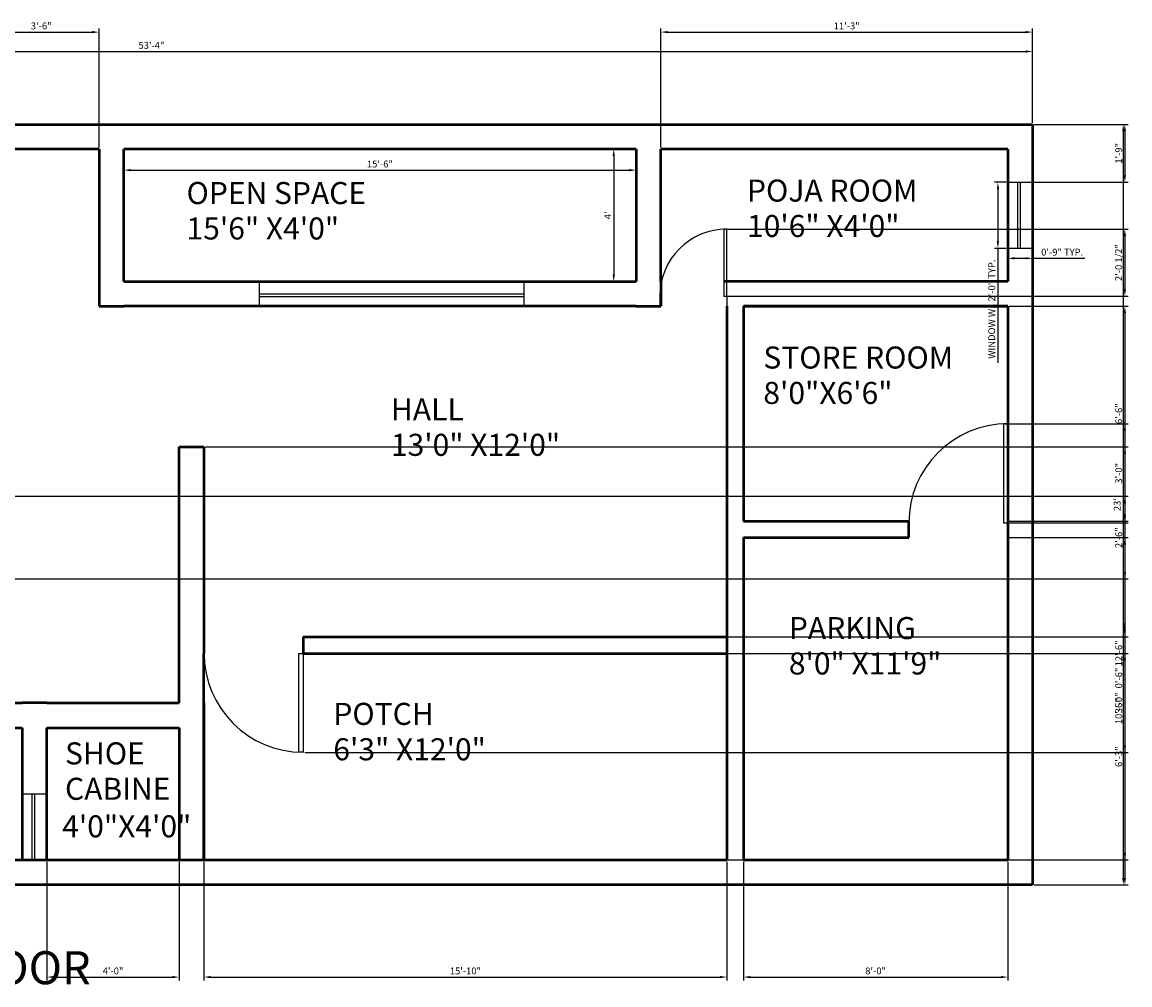
# Model space of a CAD drawing. Units: inches. Extents: x -5798 to 2718, y 1530 to 38999.
# Tile 4 of 4: x 2316 to 2718, y 1990 to 2339. Entities that reach past the tile are written whole.
import ezdxf

# ---------------------------------------------------------------- set-up
doc = ezdxf.new("R2010")
doc.units = ezdxf.units.IN
for name, color, linetype, lineweight in [('A-ANNO-DIMS', 2, 'Continuous', 18), ('A-ANNO-TEXT', 7, 'Continuous', 25), ('A-AREA-IDEN', 3, 'Continuous', 18), ('A-DOOR', 3, 'Continuous', 25), ('A-GLAZ', 4, 'Continuous', 25), ('A-WALL', 7, 'Continuous', 50)]:
    doc.layers.add(name, color=color, linetype=linetype, lineweight=lineweight)
doc.styles.get("Standard").update_dxf_attribs({"font": 'arial.ttf'})
doc.dimstyles.new('Copy of ISO-25', dxfattribs={"dimtxt": 2.5, "dimasz": 2.5, "dimexe": 1.25, "dimexo": 0.625, "dimtad": 1, "dimdec": 1, "dimlunit": 4, "dimtxsty": 'Standard', "dimcen": 2.5, "dimadec": 0, "dimazin": 0, "dimtfac": 1, "dimtdec": 1, "dimtmove": 0, "dimatfit": 3, "dimfxl": 1, "dimarcsym": 0})

# ---------------------------------------------------------------- blocks, each defined once
blk = doc.blocks.new('*U6')
for p, q in [((-40, 0), (-40, 6)), ((0, 0), (0, 6))]:
    blk.add_line(p, q)
blk.add_lwpolyline([(0, 0), (0, -40), (-1.75, -40), (-1.75, 0)], close=True)
blk.add_arc((0, 0), 40, 180, 270)
blk = doc.blocks.new('*U5')
for p, q in [((0, 0), (0, -6)), ((-40, 0), (-40, -6))]:
    blk.add_line(p, q)
blk.add_lwpolyline([(0, 0), (0, 40), (-1.75, 40), (-1.75, 0)], close=True)
blk.add_arc((0, 0), 40, 90, 180)
blk = doc.blocks.new('*D9')
at = {"layer": 'A-ANNO-DIMS', "color": 0, "lineweight": -2, "transparency": 16777216}
for p, q in [((2352.89, 2292.65), (2352.89, 2284.42)), ((2538.89, 2292.65), (2538.89, 2284.42)), ((2355.39, 2285.67), (2536.39, 2285.67))]:
    blk.add_line(p, q, dxfattribs=at)
at = {"layer": 'A-ANNO-DIMS', "color": 0, "transparency": 16777216}
for points in [[(2355.39, 2286.09), (2355.39, 2285.25), (2352.89, 2285.67)], [(2536.39, 2286.09), (2536.39, 2285.25), (2538.89, 2285.67)]]:
    blk.add_solid(points, dxfattribs=at)
at = {"layer": 'Defpoints', "color": 0, "transparency": 16777216}
for p in [(2352.89, 2293.28), (2538.89, 2293.28), (2538.89, 2285.67)]:
    blk.add_point(p, dxfattribs=at)
at = {"layer": 'A-ANNO-DIMS', "color": 0, "transparency": 16777216, "insert": (2445.89, 2287.57), "char_height": 2.5, "attachment_point": 5}
blk.add_mtext('15\'-6"', dxfattribs=at)
blk = doc.blocks.new('*D10')
at = {"layer": 'A-ANNO-DIMS', "color": 0, "lineweight": -2, "transparency": 16777216}
for p, q in [((2538.27, 2293.28), (2529.55, 2293.28)), ((2530.8, 2290.78), (2530.8, 2247.78)), ((2538.27, 2245.28), (2529.55, 2245.28))]:
    blk.add_line(p, q, dxfattribs=at)
at = {"layer": 'A-ANNO-DIMS', "color": 0, "transparency": 16777216}
for points in [[(2530.38, 2290.78), (2531.21, 2290.78), (2530.8, 2293.28)], [(2530.38, 2247.78), (2531.21, 2247.78), (2530.8, 2245.28)]]:
    blk.add_solid(points, dxfattribs=at)
at = {"layer": 'Defpoints', "color": 0, "transparency": 16777216}
for p in [(2538.89, 2293.28), (2530.8, 2245.28), (2538.89, 2245.28)]:
    blk.add_point(p, dxfattribs=at)
at = {"layer": 'A-ANNO-DIMS', "color": 0, "transparency": 16777216, "insert": (2528.92, 2269.28), "char_height": 2.5, "attachment_point": 5, "rotation": 90}
blk.add_mtext("4'", dxfattribs=at)
blk = doc.blocks.new('*D13')
at = {"layer": 'A-ANNO-DIMS', "color": 0, "lineweight": -2, "transparency": 16777216}
for p, q in [((2042.98, 2302.9), (2042.98, 2329.99)), ((2682.89, 2302.9), (2682.89, 2329.99)), ((2045.48, 2328.74), (2680.39, 2328.74))]:
    blk.add_line(p, q, dxfattribs=at)
at = {"layer": 'A-ANNO-DIMS', "color": 0, "transparency": 16777216}
for points in [[(2045.48, 2329.16), (2045.48, 2328.32), (2042.98, 2328.74)], [(2680.39, 2329.16), (2680.39, 2328.32), (2682.89, 2328.74)]]:
    blk.add_solid(points, dxfattribs=at)
at = {"layer": 'Defpoints', "color": 0, "transparency": 16777216}
for p in [(2682.89, 2328.74), (2042.98, 2302.28), (2682.89, 2302.28)]:
    blk.add_point(p, dxfattribs=at)
at = {"layer": 'A-ANNO-DIMS', "color": 0, "transparency": 16777216, "insert": (2362.93, 2330.64), "char_height": 2.5, "attachment_point": 5}
blk.add_mtext('53\'-4"', dxfattribs=at)
blk = doc.blocks.new('*D14')
at = {"layer": 'A-ANNO-DIMS', "color": 0, "lineweight": -2, "transparency": 16777216}
for p, q in [((2683.52, 2302.28), (2717.07, 2302.28)), ((2715.82, 2299.78), (2715.82, 2028.78)), ((2683.52, 2026.28), (2717.07, 2026.28))]:
    blk.add_line(p, q, dxfattribs=at)
at = {"layer": 'A-ANNO-DIMS', "color": 0, "transparency": 16777216}
for points in [[(2715.4, 2299.78), (2716.23, 2299.78), (2715.82, 2302.28)], [(2715.4, 2028.78), (2716.23, 2028.78), (2715.82, 2026.28)]]:
    blk.add_solid(points, dxfattribs=at)
at = {"layer": 'Defpoints', "color": 0, "transparency": 16777216}
for p in [(2682.89, 2302.28), (2682.89, 2026.28), (2715.82, 2026.28)]:
    blk.add_point(p, dxfattribs=at)
at = {"layer": 'A-ANNO-DIMS', "color": 0, "transparency": 16777216, "insert": (2713.92, 2164.28), "char_height": 2.5, "attachment_point": 5, "rotation": 90}
blk.add_mtext("23'", dxfattribs=at)
blk = doc.blocks.new('WIN-24')
for p, q in [((0, 0), (0, 9)), ((0, 9), (24, 9)), ((24, 9), (24, 0)), ((0, 4.5), (24, 4.5)), ((0, 3.5), (24, 3.5))]:
    blk.add_line(p, q)
blk = doc.blocks.new('*D22')
at = {"layer": 'A-ANNO-DIMS', "color": 0, "lineweight": -2, "transparency": 16777216}
for p, q in [((2673.27, 2281.28), (2669.04, 2281.28)), ((2670.29, 2278.78), (2670.29, 2259.78)), ((2673.27, 2257.28), (2669.04, 2257.28)), ((2670.29, 2257.28), (2670.29, 2215.68))]:
    blk.add_line(p, q, dxfattribs=at)
at = {"layer": 'A-ANNO-DIMS', "color": 0, "transparency": 16777216}
for points in [[(2669.88, 2278.78), (2670.71, 2278.78), (2670.29, 2281.28)], [(2669.88, 2259.78), (2670.71, 2259.78), (2670.29, 2257.28)]]:
    blk.add_solid(points, dxfattribs=at)
at = {"layer": 'Defpoints', "color": 0, "transparency": 16777216}
for p in [(2673.89, 2281.28), (2670.29, 2257.28), (2673.89, 2257.28)]:
    blk.add_point(p, dxfattribs=at)
at = {"layer": 'A-ANNO-DIMS', "color": 0, "transparency": 16777216, "insert": (2668.38, 2235.23), "char_height": 2.5, "attachment_point": 5, "rotation": 90}
blk.add_mtext('WINDOW W1 2\'-0" TYP.', dxfattribs=at)
blk = doc.blocks.new('*D23')
at = {"layer": 'A-ANNO-DIMS', "color": 0, "lineweight": -2, "transparency": 16777216}
for p, q in [((2673.89, 2256.65), (2673.89, 2252.43)), ((2682.89, 2256.65), (2682.89, 2252.43)), ((2676.39, 2253.68), (2680.39, 2253.68)), ((2682.89, 2253.68), (2701.88, 2253.68))]:
    blk.add_line(p, q, dxfattribs=at)
at = {"layer": 'A-ANNO-DIMS', "color": 0, "transparency": 16777216}
for points in [[(2676.39, 2254.09), (2676.39, 2253.26), (2673.89, 2253.68)], [(2680.39, 2254.09), (2680.39, 2253.26), (2682.89, 2253.68)]]:
    blk.add_solid(points, dxfattribs=at)
at = {"layer": 'Defpoints', "color": 0, "transparency": 16777216}
for p in [(2673.89, 2257.28), (2682.89, 2257.28), (2682.89, 2253.68)]:
    blk.add_point(p, dxfattribs=at)
at = {"layer": 'A-ANNO-DIMS', "color": 0, "transparency": 16777216, "insert": (2693.64, 2255.58), "char_height": 2.5, "attachment_point": 5}
blk.add_mtext('0\'-9" TYP.', dxfattribs=at)
blk = doc.blocks.new('*D37')
at = {"layer": 'A-ANNO-DIMS', "color": 0, "lineweight": -2, "transparency": 16777216}
for p, q in [((2301.89, 2293.9), (2301.89, 2337.03)), ((2343.89, 2293.9), (2343.89, 2337.03)), ((2304.39, 2335.78), (2341.39, 2335.78))]:
    blk.add_line(p, q, dxfattribs=at)
at = {"layer": 'A-ANNO-DIMS', "color": 0, "transparency": 16777216}
for points in [[(2304.39, 2336.19), (2304.39, 2335.36), (2301.89, 2335.78)], [(2341.39, 2336.19), (2341.39, 2335.36), (2343.89, 2335.78)]]:
    blk.add_solid(points, dxfattribs=at)
at = {"layer": 'Defpoints', "color": 0, "transparency": 16777216}
for p in [(2343.89, 2335.78), (2301.89, 2293.28), (2343.89, 2293.28)]:
    blk.add_point(p, dxfattribs=at)
at = {"layer": 'A-ANNO-DIMS', "color": 0, "transparency": 16777216, "insert": (2322.89, 2337.68), "char_height": 2.5, "attachment_point": 5}
blk.add_mtext('3\'-6"', dxfattribs=at)
blk = doc.blocks.new('*D38')
at = {"layer": 'A-ANNO-DIMS', "color": 0, "lineweight": -2, "transparency": 16777216}
for p, q in [((2547.89, 2293.9), (2547.89, 2337.03)), ((2682.89, 2302.9), (2682.89, 2337.03)), ((2550.39, 2335.78), (2680.39, 2335.78))]:
    blk.add_line(p, q, dxfattribs=at)
at = {"layer": 'A-ANNO-DIMS', "color": 0, "transparency": 16777216}
for points in [[(2550.39, 2336.19), (2550.39, 2335.36), (2547.89, 2335.78)], [(2680.39, 2336.19), (2680.39, 2335.36), (2682.89, 2335.78)]]:
    blk.add_solid(points, dxfattribs=at)
at = {"layer": 'Defpoints', "color": 0, "transparency": 16777216}
for p in [(2682.89, 2335.78), (2682.89, 2302.28), (2547.89, 2293.28)]:
    blk.add_point(p, dxfattribs=at)
at = {"layer": 'A-ANNO-DIMS', "color": 0, "transparency": 16777216, "insert": (2615.39, 2337.68), "char_height": 2.5, "attachment_point": 5}
blk.add_mtext('11\'-3"', dxfattribs=at)
blk = doc.blocks.new('*D44')
at = {"layer": 'A-ANNO-DIMS', "color": 0, "lineweight": -2, "transparency": 16777216}
for p, q in [((2683.52, 2302.28), (2717.64, 2302.28)), ((2716.39, 2299.78), (2716.39, 2283.78)), ((2683.52, 2281.28), (2717.64, 2281.28))]:
    blk.add_line(p, q, dxfattribs=at)
at = {"layer": 'A-ANNO-DIMS', "color": 0, "transparency": 16777216}
for points in [[(2715.98, 2299.78), (2716.81, 2299.78), (2716.39, 2302.28)], [(2715.98, 2283.78), (2716.81, 2283.78), (2716.39, 2281.28)]]:
    blk.add_solid(points, dxfattribs=at)
at = {"layer": 'Defpoints', "color": 0, "transparency": 16777216}
for p in [(2682.89, 2302.28), (2682.89, 2281.28), (2716.39, 2281.28)]:
    blk.add_point(p, dxfattribs=at)
at = {"layer": 'A-ANNO-DIMS', "color": 0, "transparency": 16777216, "insert": (2714.49, 2291.78), "char_height": 2.5, "attachment_point": 5, "rotation": 90}
blk.add_mtext('1\'-9"', dxfattribs=at)
blk = doc.blocks.new('*D45')
at = {"layer": 'A-ANNO-DIMS', "color": 0, "lineweight": -2, "transparency": 16777216}
for p, q in [((2674.52, 2236.28), (2717.64, 2236.28)), ((2716.39, 2233.78), (2716.39, 2160.78)), ((2674.52, 2158.28), (2717.64, 2158.28))]:
    blk.add_line(p, q, dxfattribs=at)
at = {"layer": 'A-ANNO-DIMS', "color": 0, "transparency": 16777216}
for points in [[(2715.98, 2233.78), (2716.81, 2233.78), (2716.39, 2236.28)], [(2715.98, 2160.78), (2716.81, 2160.78), (2716.39, 2158.28)]]:
    blk.add_solid(points, dxfattribs=at)
at = {"layer": 'Defpoints', "color": 0, "transparency": 16777216}
for p in [(2673.89, 2236.28), (2673.89, 2158.28), (2716.39, 2158.28)]:
    blk.add_point(p, dxfattribs=at)
at = {"layer": 'A-ANNO-DIMS', "color": 0, "transparency": 16777216, "insert": (2714.49, 2197.28), "char_height": 2.5, "attachment_point": 5, "rotation": 90}
blk.add_mtext('6\'-6"', dxfattribs=at)
blk = doc.blocks.new('*D46')
at = {"layer": 'A-ANNO-DIMS', "color": 0, "lineweight": -2, "transparency": 16777216}
for p, q in [((2674.52, 2152.28), (2717.64, 2152.28)), ((2716.39, 2149.78), (2716.39, 2028.78)), ((2683.52, 2026.28), (2717.64, 2026.28))]:
    blk.add_line(p, q, dxfattribs=at)
at = {"layer": 'A-ANNO-DIMS', "color": 0, "transparency": 16777216}
for points in [[(2715.98, 2149.78), (2716.81, 2149.78), (2716.39, 2152.28)], [(2715.98, 2028.78), (2716.81, 2028.78), (2716.39, 2026.28)]]:
    blk.add_solid(points, dxfattribs=at)
at = {"layer": 'Defpoints', "color": 0, "transparency": 16777216}
for p in [(2673.89, 2152.28), (2682.89, 2026.28), (2716.39, 2026.28)]:
    blk.add_point(p, dxfattribs=at)
at = {"layer": 'A-ANNO-DIMS', "color": 0, "transparency": 16777216, "insert": (2714.49, 2089.28), "char_height": 2.5, "attachment_point": 5, "rotation": 90}
blk.add_mtext('10\'-6"', dxfattribs=at)
blk = doc.blocks.new('*D50')
at = {"layer": 'A-ANNO-DIMS', "color": 0, "lineweight": -2, "transparency": 16777216}
for p, q in [((2324.98, 2034.65), (2324.98, 1991.53)), ((2372.98, 2034.65), (2372.98, 1991.53)), ((2327.48, 1992.78), (2370.48, 1992.78))]:
    blk.add_line(p, q, dxfattribs=at)
at = {"layer": 'A-ANNO-DIMS', "color": 0, "transparency": 16777216}
for points in [[(2327.48, 1993.19), (2327.48, 1992.36), (2324.98, 1992.78)], [(2370.48, 1993.19), (2370.48, 1992.36), (2372.98, 1992.78)]]:
    blk.add_solid(points, dxfattribs=at)
at = {"layer": 'Defpoints', "color": 0, "transparency": 16777216}
for p in [(2324.98, 2035.28), (2372.98, 2035.28), (2372.98, 1992.78)]:
    blk.add_point(p, dxfattribs=at)
at = {"layer": 'A-ANNO-DIMS', "color": 0, "transparency": 16777216, "insert": (2348.98, 1994.68), "char_height": 2.5, "attachment_point": 5}
blk.add_mtext('4\'-0"', dxfattribs=at)
blk = doc.blocks.new('*D51')
at = {"layer": 'A-ANNO-DIMS', "color": 0, "lineweight": -2, "transparency": 16777216}
for p, q in [((2381.98, 2034.65), (2381.98, 1991.53)), ((2571.89, 2034.65), (2571.89, 1991.53)), ((2384.48, 1992.78), (2569.39, 1992.78))]:
    blk.add_line(p, q, dxfattribs=at)
at = {"layer": 'A-ANNO-DIMS', "color": 0, "transparency": 16777216}
for points in [[(2384.48, 1993.19), (2384.48, 1992.36), (2381.98, 1992.78)], [(2569.39, 1993.19), (2569.39, 1992.36), (2571.89, 1992.78)]]:
    blk.add_solid(points, dxfattribs=at)
at = {"layer": 'Defpoints', "color": 0, "transparency": 16777216}
for p in [(2381.98, 2035.28), (2571.89, 2035.28), (2571.89, 1992.78)]:
    blk.add_point(p, dxfattribs=at)
at = {"layer": 'A-ANNO-DIMS', "color": 0, "transparency": 16777216, "insert": (2476.93, 1994.68), "char_height": 2.5, "attachment_point": 5}
blk.add_mtext('15\'-10"', dxfattribs=at)
blk = doc.blocks.new('*D52')
at = {"layer": 'A-ANNO-DIMS', "color": 0, "lineweight": -2, "transparency": 16777216}
for p, q in [((2577.89, 2034.65), (2577.89, 1991.53)), ((2673.89, 2034.65), (2673.89, 1991.53)), ((2580.39, 1992.78), (2671.39, 1992.78))]:
    blk.add_line(p, q, dxfattribs=at)
at = {"layer": 'A-ANNO-DIMS', "color": 0, "transparency": 16777216}
for points in [[(2580.39, 1993.19), (2580.39, 1992.36), (2577.89, 1992.78)], [(2671.39, 1993.19), (2671.39, 1992.36), (2673.89, 1992.78)]]:
    blk.add_solid(points, dxfattribs=at)
at = {"layer": 'Defpoints', "color": 0, "transparency": 16777216}
for p in [(2577.89, 2035.28), (2673.89, 2035.28), (2673.89, 1992.78)]:
    blk.add_point(p, dxfattribs=at)
at = {"layer": 'A-ANNO-DIMS', "color": 0, "transparency": 16777216, "insert": (2625.89, 1994.68), "char_height": 2.5, "attachment_point": 5}
blk.add_mtext('8\'-0"', dxfattribs=at)
blk = doc.blocks.new('*D55')
at = {"layer": 'A-ANNO-DIMS', "color": 0, "lineweight": -2, "transparency": 16777216}
for p, q in [((2382.6, 2185.28), (2717.64, 2185.28)), ((2716.39, 2182.78), (2716.39, 2037.78)), ((2382.6, 2035.28), (2717.64, 2035.28))]:
    blk.add_line(p, q, dxfattribs=at)
at = {"layer": 'A-ANNO-DIMS', "color": 0, "transparency": 16777216}
for points in [[(2715.98, 2182.78), (2716.81, 2182.78), (2716.39, 2185.28)], [(2715.98, 2037.78), (2716.81, 2037.78), (2716.39, 2035.28)]]:
    blk.add_solid(points, dxfattribs=at)
at = {"layer": 'Defpoints', "color": 0, "transparency": 16777216}
for p in [(2381.98, 2185.28), (2381.98, 2035.28), (2716.39, 2035.28)]:
    blk.add_point(p, dxfattribs=at)
at = {"layer": 'A-ANNO-DIMS', "color": 0, "transparency": 16777216, "insert": (2714.49, 2110.28), "char_height": 2.5, "attachment_point": 5, "rotation": 90}
blk.add_mtext('12\'-6"', dxfattribs=at)
blk = doc.blocks.new('*D56')
at = {"layer": 'A-ANNO-DIMS', "color": 0, "lineweight": -2, "transparency": 16777216}
for p, q in [((2572.52, 2110.28), (2717.64, 2110.28)), ((2716.39, 2107.78), (2716.39, 2037.78)), ((2572.52, 2035.28), (2717.64, 2035.28))]:
    blk.add_line(p, q, dxfattribs=at)
at = {"layer": 'A-ANNO-DIMS', "color": 0, "transparency": 16777216}
for points in [[(2715.98, 2107.78), (2716.81, 2107.78), (2716.39, 2110.28)], [(2715.98, 2037.78), (2716.81, 2037.78), (2716.39, 2035.28)]]:
    blk.add_solid(points, dxfattribs=at)
at = {"layer": 'Defpoints', "color": 0, "transparency": 16777216}
for p in [(2571.89, 2110.28), (2571.89, 2035.28), (2716.39, 2035.28)]:
    blk.add_point(p, dxfattribs=at)
at = {"layer": 'A-ANNO-DIMS', "color": 0, "transparency": 16777216, "insert": (2714.49, 2072.78), "char_height": 2.5, "attachment_point": 5, "rotation": 90}
blk.add_mtext('6\'-3"', dxfattribs=at)
blk = doc.blocks.new('*D57')
at = {"layer": 'A-ANNO-DIMS', "color": 0, "lineweight": -2, "transparency": 16777216}
for p, q in [((2716.39, 2118.78), (2716.39, 2121.28)), ((2418.6, 2116.28), (2717.64, 2116.28)), ((2716.39, 2116.28), (2716.39, 2110.28)), ((2418.6, 2110.28), (2717.64, 2110.28)), ((2716.39, 2107.78), (2716.39, 2097.38))]:
    blk.add_line(p, q, dxfattribs=at)
at = {"layer": 'A-ANNO-DIMS', "color": 0, "transparency": 16777216}
for points in [[(2715.98, 2118.78), (2716.81, 2118.78), (2716.39, 2116.28)], [(2715.98, 2107.78), (2716.81, 2107.78), (2716.39, 2110.28)]]:
    blk.add_solid(points, dxfattribs=at)
at = {"layer": 'Defpoints', "color": 0, "transparency": 16777216}
for p in [(2417.98, 2116.28), (2417.98, 2110.28), (2716.39, 2110.28)]:
    blk.add_point(p, dxfattribs=at)
at = {"layer": 'A-ANNO-DIMS', "color": 0, "transparency": 16777216, "insert": (2714.49, 2101.33), "char_height": 2.5, "attachment_point": 5, "rotation": 90}
blk.add_mtext('0\'-6"', dxfattribs=at)
blk = doc.blocks.new('*D59')
at = {"layer": 'A-ANNO-DIMS', "color": 0, "lineweight": -2, "transparency": 16777216}
for p, q in [((2181.6, 2167.28), (2717.64, 2167.28)), ((2716.39, 2164.78), (2716.39, 2139.78)), ((2181.6, 2137.28), (2717.64, 2137.28))]:
    blk.add_line(p, q, dxfattribs=at)
at = {"layer": 'A-ANNO-DIMS', "color": 0, "transparency": 16777216}
for points in [[(2715.98, 2164.78), (2716.81, 2164.78), (2716.39, 2167.28)], [(2715.98, 2139.78), (2716.81, 2139.78), (2716.39, 2137.28)]]:
    blk.add_solid(points, dxfattribs=at)
at = {"layer": 'Defpoints', "color": 0, "transparency": 16777216}
for p in [(2180.98, 2167.28), (2180.98, 2137.28), (2716.39, 2137.28)]:
    blk.add_point(p, dxfattribs=at)
at = {"layer": 'A-ANNO-DIMS', "color": 0, "transparency": 16777216, "insert": (2714.49, 2152.28), "char_height": 2.5, "attachment_point": 5, "rotation": 90}
blk.add_mtext('2\'-6"', dxfattribs=at)
blk = doc.blocks.new('*D62')
at = {"layer": 'A-ANNO-DIMS', "color": 0, "lineweight": -2, "transparency": 16777216}
for p, q in [((2418.6, 2110.28), (2717.64, 2110.28)), ((2716.39, 2107.78), (2716.39, 2076.85)), ((2418.6, 2074.35), (2717.64, 2074.35))]:
    blk.add_line(p, q, dxfattribs=at)
at = {"layer": 'A-ANNO-DIMS', "color": 0, "transparency": 16777216}
for points in [[(2715.98, 2107.78), (2716.81, 2107.78), (2716.39, 2110.28)], [(2715.98, 2076.85), (2716.81, 2076.85), (2716.39, 2074.35)]]:
    blk.add_solid(points, dxfattribs=at)
at = {"layer": 'Defpoints', "color": 0, "transparency": 16777216}
for p in [(2417.98, 2110.28), (2417.98, 2074.35), (2716.39, 2074.35)]:
    blk.add_point(p, dxfattribs=at)
at = {"layer": 'A-ANNO-DIMS', "color": 0, "transparency": 16777216, "insert": (2714.49, 2092.32), "char_height": 2.5, "attachment_point": 5, "rotation": 90}
blk.add_mtext('3\'-0"', dxfattribs=at)
blk = doc.blocks.new('*D63')
at = {"layer": 'A-ANNO-DIMS', "color": 0, "lineweight": -2, "transparency": 16777216}
for p, q in [((2571.45, 2264.3), (2717.64, 2264.3)), ((2716.39, 2261.8), (2716.39, 2242.43)), ((2571.45, 2239.93), (2717.64, 2239.93))]:
    blk.add_line(p, q, dxfattribs=at)
at = {"layer": 'A-ANNO-DIMS', "color": 0, "transparency": 16777216}
for points in [[(2715.98, 2261.8), (2716.81, 2261.8), (2716.39, 2264.3)], [(2715.98, 2242.43), (2716.81, 2242.43), (2716.39, 2239.93)]]:
    blk.add_solid(points, dxfattribs=at)
at = {"layer": 'Defpoints', "color": 0, "transparency": 16777216}
for p in [(2570.83, 2264.3), (2570.83, 2239.93), (2716.39, 2239.93)]:
    blk.add_point(p, dxfattribs=at)
at = {"layer": 'A-ANNO-DIMS', "color": 0, "transparency": 16777216, "insert": (2714.48, 2252.12), "char_height": 2.5, "attachment_point": 5, "rotation": 90}
blk.add_mtext('2\'-0 1/2"', dxfattribs=at)
blk = doc.blocks.new('*D64')
at = {"layer": 'A-ANNO-DIMS', "color": 0, "lineweight": -2, "transparency": 16777216}
for p, q in [((2672.95, 2193.59), (2717.64, 2193.59)), ((2716.39, 2191.09), (2716.39, 2160.17)), ((2672.95, 2157.67), (2717.64, 2157.67))]:
    blk.add_line(p, q, dxfattribs=at)
at = {"layer": 'A-ANNO-DIMS', "color": 0, "transparency": 16777216}
for points in [[(2715.98, 2191.09), (2716.81, 2191.09), (2716.39, 2193.59)], [(2715.98, 2160.17), (2716.81, 2160.17), (2716.39, 2157.67)]]:
    blk.add_solid(points, dxfattribs=at)
at = {"layer": 'Defpoints', "color": 0, "transparency": 16777216}
for p in [(2672.32, 2193.59), (2672.32, 2157.67), (2716.39, 2157.67)]:
    blk.add_point(p, dxfattribs=at)
at = {"layer": 'A-ANNO-DIMS', "color": 0, "transparency": 16777216, "insert": (2714.49, 2175.63), "char_height": 2.5, "attachment_point": 5, "rotation": 90}
blk.add_mtext('3\'-0"', dxfattribs=at)

msp = doc.modelspace()

# ---------------------------------------------------------------- linework, layer by layer
at = {"layer": 'A-GLAZ'}
for p, q in [((2402.14, 2236.28), (2402.14, 2245.28)), ((2498.14, 2245.28), (2498.14, 2236.28)), ((2402.14, 2240.78), (2498.14, 2240.78)), ((2402.14, 2239.78), (2498.14, 2239.78)), ((2498.14, 2236.28), (2402.14, 2236.28))]:
    msp.add_line(p, q, dxfattribs=at)
at = {"layer": 'A-WALL'}
for p, q in [((2301.89, 2302.28), (2541.89, 2302.28)), ((2541.89, 2302.28), (2547.89, 2302.28)), ((2547.89, 2302.28), (2673.89, 2302.28)), ((2673.89, 2302.28), (2682.89, 2302.28)), ((2682.89, 2302.28), (2682.89, 2293.28)), ((2343.89, 2293.28), (2301.89, 2293.28)), ((2343.89, 2293.28), (2343.89, 2245.28)), ((2352.89, 2245.28), (2352.89, 2293.28)), ((2538.89, 2293.28), (2352.89, 2293.28)), ((2538.89, 2293.28), (2538.89, 2245.28)), ((2673.89, 2293.28), (2547.89, 2293.28)), ((2547.89, 2245.28), (2547.89, 2293.28)), ((2673.89, 2293.28), (2673.89, 2245.28)), ((2673.89, 2293.28), (2673.89, 2245.28)), ((2673.89, 2293.28), (2673.89, 2281.28)), ((2682.89, 2293.28), (2682.89, 2245.28)), ((2343.89, 2245.28), (2343.89, 2236.28)), ((2352.89, 2245.28), (2538.89, 2245.28)), ((2498.14, 2245.28), (2498.14, 2245.28)), ((2547.89, 2245.28), (2547.89, 2236.28)), ((2548.12, 2245.28), (2547.89, 2245.28)), ((2673.89, 2245.28), (2570.83, 2245.28)), ((2682.89, 2245.28), (2682.89, 2239.28)), ((2682.89, 2239.28), (2682.89, 2161.28)), ((2343.89, 2236.28), (2352.89, 2236.28)), ((2538.89, 2236.28), (2352.89, 2236.28)), ((2538.89, 2236.28), (2547.89, 2236.28)), ((2571.89, 2236.28), (2571.89, 2158.28)), ((2673.89, 2236.28), (2577.89, 2236.28)), ((2577.89, 2236.28), (2577.89, 2158.28)), ((2577.89, 2236.28), (2673.89, 2236.28)), ((2673.89, 2236.28), (2673.89, 2158.28)), ((2372.98, 2092.28), (2372.98, 2185.28)), ((2372.98, 2185.28), (2381.98, 2185.28)), ((2381.98, 2185.28), (2381.98, 2116.28)), ((2682.89, 2161.28), (2682.89, 2155.28)), ((2571.89, 2158.28), (2571.89, 2152.28)), ((2577.89, 2158.28), (2637.89, 2158.28)), ((2637.89, 2152.28), (2637.89, 2158.28)), ((2673.89, 2158.28), (2673.89, 2152.28)), ((2571.89, 2152.28), (2571.89, 2035.28)), ((2577.89, 2152.28), (2637.89, 2152.28)), ((2577.89, 2152.28), (2577.89, 2035.28)), ((2673.89, 2152.28), (2673.89, 2035.28)), ((2682.89, 2155.28), (2682.89, 2026.28)), ((2381.98, 2118.51), (2381.98, 2118.51)), ((2381.98, 2118.51), (2381.98, 2110.28)), ((2417.98, 2116.28), (2571.89, 2116.28)), ((2417.98, 2116.28), (2417.98, 2110.28)), ((2381.98, 2035.28), (2381.98, 2110.28)), ((2417.98, 2110.28), (2571.89, 2110.28)), ((2278.97, 2092.28), (2315.98, 2092.28)), ((2324.98, 2092.28), (2315.98, 2092.28)), ((2324.98, 2092.28), (2372.98, 2092.28)), ((2381.98, 2092.28), (2381.98, 2035.28)), ((2381.98, 2035.28), (2381.98, 2092.28)), ((2278.97, 2083.28), (2315.98, 2083.28)), ((2315.98, 2083.28), (2315.98, 2035.28)), ((2324.98, 2035.28), (2324.98, 2083.28)), ((2324.98, 2083.28), (2372.98, 2083.28)), ((2372.98, 2083.28), (2372.98, 2035.28)), ((2051.98, 2035.28), (2571.89, 2035.28)), ((2372.98, 2035.28), (2381.98, 2035.28)), ((2577.89, 2035.28), (2673.89, 2035.28)), ((2682.89, 2035.28), (2682.89, 2026.28)), ((2682.89, 2026.28), (2042.98, 2026.28))]:
    msp.add_line(p, q, dxfattribs=at)

# ---------------------------------------------------------------- block references
at = {"layer": 'A-DOOR'}
for name, p, xscale, yscale, zscale in [('*U5', (2571.89, 2239.93), 0.6091863517261157, 0.6091863517261157, 0.6091863517261157), ('*U5', (2673.89, 2157.67), 0.8981214444059173, 0.8981214444059173, 0.8981214444059173), ('*U5', (2673.89, 2157.67), 0.8981214444059173, 0.8981214444059173, 0.8981214444059173), ('*U6', (2417.98, 2110.28), 0.8981214444059173, 0.8981214444059173, 0.8981214444059173)]:
    msp.add_blockref(name, p, dxfattribs=dict(at, xscale=xscale, yscale=yscale, zscale=zscale))
at = {"layer": 'A-GLAZ'}
for p, rotation in [((2673.89, 2281.28), 270.0000000000009), ((2315.98, 2059.28), 269.9999999999973)]:
    msp.add_blockref('WIN-24', p, dxfattribs=dict(at, rotation=rotation))

# ---------------------------------------------------------------- texts
at = {"layer": 'A-ANNO-TEXT'}
msp.add_text('GROUND FLOOR ', height=12, dxfattribs=at).set_placement((2215.86, 1990.17))
at = {"layer": 'A-AREA-IDEN'}
for s, p in [('OPEN SPACE', (2375.66, 2273.36)), ('POJA ROOM', (2579.18, 2274.25)), ('15\'6" X4\'0"', (2375.66, 2260.5)), ('10\'6" X4\'0"', (2579.18, 2261.4)), ('STORE ROOM', (2585.12, 2213.65)), ('8\'0"X6\'6"', (2585.12, 2200.8)), ('HALL', (2449.88, 2194.82)), ('13\'0" X12\'0"', (2449.88, 2181.97)), ('PARKING', (2594.38, 2115.46)), ('8\'0" X11\'9"', (2594.38, 2102.61)), ('POTCH', (2428.97, 2084.31)), ('6\'3" X12\'0"', (2428.97, 2071.46)), ('SHOE', (2331.54, 2069.97)), ('CABINE', (2331.54, 2057.12)), ('4\'0"X4\'0"', (2330.51, 2043.49))]:
    msp.add_text(s, height=8, dxfattribs=at).set_placement(p)

# ---------------------------------------------------------------- dimensions: what is measured, and where the dimension line sits
at = {"layer": 'A-ANNO-DIMS'}
for base, p1, p2, override, picture, middle in [((2343.89, 2335.78), (2301.89, 2293.28), (2343.89, 2293.28), {"dimdec": 1, "dimlfac": 1, "dimrnd": 0, "dimzin": 1, "dimdsep": 46, "dimlunit": 4, "dimfrac": 2}, '*D37', (2322.89, 2337.68)), ((2682.89, 2335.78), (2547.89, 2293.28), (2682.89, 2302.28), {"dimdec": 1, "dimlfac": 1, "dimrnd": 0, "dimzin": 1, "dimdsep": 46, "dimlunit": 4, "dimfrac": 2}, '*D38', (2615.39, 2337.68)), ((2682.89, 2328.74), (2042.98, 2302.28), (2682.89, 2302.28), {"dimclrd": 0, "dimclre": 0, "dimclrt": 0}, '*D13', (2362.93, 2330.64)), ((2538.89, 2285.67), (2352.89, 2293.28), (2538.89, 2293.28), {"dimclrd": 0, "dimclre": 0, "dimclrt": 0}, '*D9', (2445.89, 2287.57)), ((2372.98, 1992.78), (2324.98, 2035.28), (2372.98, 2035.28), {"dimdec": 1, "dimlfac": 1, "dimrnd": 0, "dimzin": 1, "dimdsep": 46, "dimlunit": 4, "dimfrac": 2}, '*D50', (2348.98, 1994.68)), ((2571.89, 1992.78), (2381.98, 2035.28), (2571.89, 2035.28), {"dimdec": 1, "dimlfac": 1, "dimrnd": 0, "dimzin": 1, "dimdsep": 46, "dimlunit": 4, "dimfrac": 2}, '*D51', (2476.93, 1994.68)), ((2673.89, 1992.78), (2577.89, 2035.28), (2673.89, 2035.28), {"dimdec": 1, "dimlfac": 1, "dimrnd": 0, "dimzin": 1, "dimdsep": 46, "dimlunit": 4, "dimfrac": 2}, '*D52', (2625.89, 1994.68))]:
    dim = msp.add_linear_dim(base=base, p1=p1, p2=p2, dimstyle='Copy of ISO-25', override=override, dxfattribs=at)
    dim.commit()
    dim.dimension.update_dxf_attribs({"geometry": picture, "text_midpoint": middle})
for base, p1, p2, override, picture, middle in [((2715.82, 2026.28), (2682.89, 2302.28), (2682.89, 2026.28), {"dimclrd": 0, "dimclre": 0, "dimclrt": 0}, '*D14', (2713.92, 2164.28)), ((2716.39, 2281.28), (2682.89, 2302.28), (2682.89, 2281.28), {"dimdec": 1, "dimlfac": 1, "dimrnd": 0, "dimzin": 1, "dimdsep": 46, "dimlunit": 4, "dimfrac": 2}, '*D44', (2714.49, 2291.78)), ((2530.8, 2245.28), (2538.89, 2293.28), (2538.89, 2245.28), {"dimclrd": 0, "dimclre": 0, "dimclrt": 0}, '*D10', (2528.92, 2269.28)), ((2716.39, 2239.93), (2570.83, 2264.3), (2570.83, 2239.93), {"dimdec": 1, "dimlfac": 1, "dimrnd": 0, "dimzin": 1, "dimdsep": 46, "dimlunit": 4, "dimfrac": 2}, '*D63', (2714.48, 2252.12)), ((2716.39, 2158.28), (2673.89, 2236.28), (2673.89, 2158.28), {"dimdec": 1, "dimlfac": 1, "dimrnd": 0, "dimzin": 1, "dimdsep": 46, "dimlunit": 4, "dimfrac": 2}, '*D45', (2714.49, 2197.28)), ((2716.39, 2157.67), (2672.32, 2193.59), (2672.32, 2157.67), {"dimdec": 1, "dimlfac": 1, "dimrnd": 0, "dimzin": 1, "dimdsep": 46, "dimlunit": 4, "dimfrac": 2}, '*D64', (2714.49, 2175.63)), ((2716.39, 2035.28), (2381.98, 2185.28), (2381.98, 2035.28), {"dimdec": 1, "dimlfac": 1, "dimrnd": 0, "dimzin": 1, "dimdsep": 46, "dimlunit": 4, "dimfrac": 2}, '*D55', (2714.49, 2110.28)), ((2716.39, 2137.28), (2180.98, 2167.28), (2180.98, 2137.28), {"dimdec": 1, "dimlfac": 1, "dimrnd": 0, "dimzin": 1, "dimdsep": 46, "dimlunit": 4, "dimfrac": 2}, '*D59', (2714.49, 2152.28)), ((2716.39, 2026.28), (2673.89, 2152.28), (2682.89, 2026.28), {"dimdec": 1, "dimlfac": 1, "dimrnd": 0, "dimzin": 1, "dimdsep": 46, "dimlunit": 4, "dimfrac": 2}, '*D46', (2714.49, 2089.28)), ((2716.39, 2110.28), (2417.98, 2116.28), (2417.98, 2110.28), {"dimdec": 1, "dimlfac": 1, "dimrnd": 0, "dimzin": 1, "dimdsep": 46, "dimlunit": 4, "dimfrac": 2}, '*D57', (2714.49, 2101.33)), ((2716.39, 2074.35), (2417.98, 2110.28), (2417.98, 2074.35), {"dimdec": 1, "dimlfac": 1, "dimrnd": 0, "dimzin": 1, "dimdsep": 46, "dimlunit": 4, "dimfrac": 2}, '*D62', (2714.49, 2092.32)), ((2716.39, 2035.28), (2571.89, 2110.28), (2571.89, 2035.28), {"dimdec": 1, "dimlfac": 1, "dimrnd": 0, "dimzin": 1, "dimdsep": 46, "dimlunit": 4, "dimfrac": 2}, '*D56', (2714.49, 2072.78))]:
    dim = msp.add_linear_dim(base=base, p1=p1, p2=p2, angle=90, dimstyle='Copy of ISO-25', override=override, dxfattribs=at)
    dim.commit()
    dim.dimension.update_dxf_attribs({"geometry": picture, "text_midpoint": middle})
dim = msp.add_linear_dim(base=(2670.29, 2257.28), p1=(2673.89, 2281.28), p2=(2673.89, 2257.28), angle=270, text='WINDOW W1 <> TYP.', dimstyle='Copy of ISO-25', override={"dimdec": 1, "dimrnd": 0, "dimzin": 1, "dimlunit": 4, "dimfrac": 2}, dxfattribs=at)
dim.commit()
dim.dimension.update_dxf_attribs({"geometry": '*D22', "text_midpoint": (2668.38, 2235.23)})
dim = msp.add_linear_dim(base=(2682.89, 2253.68), p1=(2673.89, 2257.28), p2=(2682.89, 2257.28), text='<> TYP.', dimstyle='Copy of ISO-25', override={"dimdec": 1, "dimrnd": 0, "dimzin": 1, "dimlunit": 4, "dimfrac": 2}, dxfattribs=at)
dim.commit()
dim.dimension.update_dxf_attribs({"geometry": '*D23', "text_midpoint": (2693.64, 2255.58)})

doc.saveas('drawing.dxf')
